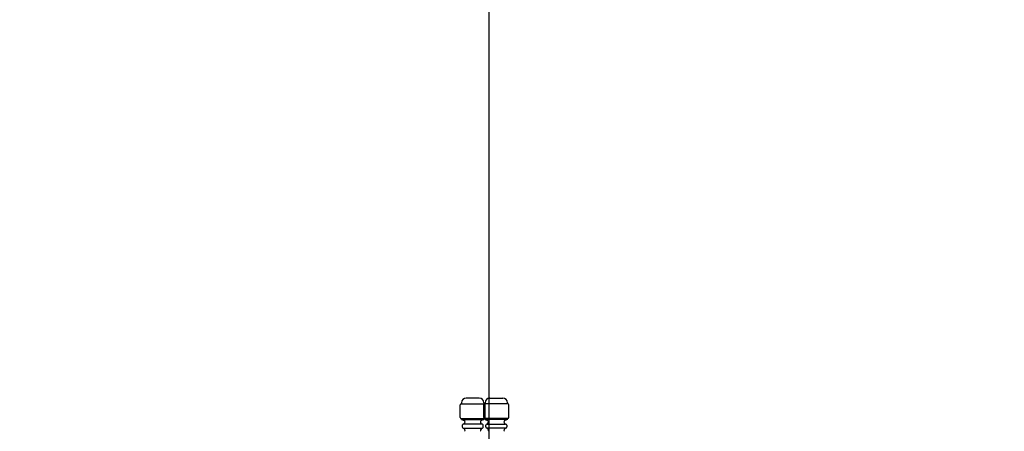
# Model space of a CAD drawing. Units: inches. Extents: x 2278 to 7495, y -71 to 1198.
# Tile 15 of 44: x 4938 to 5007, y 162 to 191. Entities that reach past the tile are written whole.
import ezdxf

# ---------------------------------------------------------------- set-up
doc = ezdxf.new("R2010")
doc.units = ezdxf.units.IN
doc.header["$MEASUREMENT"] = 0
doc.layers.add('A-ANNO-DIMS', color=2, linetype='Continuous', lineweight=18)
doc.layers.add('A-ELEV', color=7, linetype='Continuous', lineweight=25)
doc.styles.get("Standard").update_dxf_attribs({"font": 'arial.ttf'})
doc.dimstyles.get("Standard").update_dxf_attribs({"dimtxt": 6, "dimasz": 3, "dimexe": 0.18, "dimexo": 0.0625, "dimgap": 0.09, "dimtad": 0, "dimtih": 1, "dimtoh": 1, "dimdec": 0, "dimzin": 0, "dimdsep": 46, "dimlunit": 3, "dimtxsty": 'Standard', "dimblk": 'ARCHTICK', "dimcen": 0.09, "dimadec": 0, "dimazin": 0, "dimtfac": 1, "dimtdec": 0, "dimtofl": 0, "dimtmove": 0, "dimatfit": 3, "dimfxl": 1, "dimtolj": 1, "dimtzin": 0, "dimarcsym": 0})

# ---------------------------------------------------------------- blocks, each defined once
blk = doc.blocks.new('_ArchTick')
at = {"color": 0, "linetype": 'ByBlock', "const_width": 0.15}
blk.add_lwpolyline([(-0.5, -0.5), (0.5, 0.5)], dxfattribs=at)
blk = doc.blocks.new('*D123')
at = {"layer": 'A-ANNO-DIMS', "color": 0, "lineweight": -2, "transparency": 16777216}
for p, q in [((4736.95, 340.157), (4736.95, -23.427)), ((5145.676, -1.81), (5145.676, -23.427)), ((4736.95, -23.247), (4923.929, -23.247)), ((5145.676, -23.247), (4958.697, -23.247))]:
    blk.add_line(p, q, dxfattribs=at)
at = {"layer": 'Defpoints', "color": 0, "transparency": 16777216}
for p in [(4736.95, 340.219), (5145.676, -1.747), (5145.676, -23.247)]:
    blk.add_point(p, dxfattribs=at)
at = {"layer": 'A-ANNO-DIMS', "color": 0, "lineweight": -2, "transparency": 16777216, "xscale": 3, "yscale": 3, "zscale": 3, "rotation": 180}
blk.add_blockref('_ArchTick', (4736.95, -23.247), dxfattribs=at)
at = {"layer": 'A-ANNO-DIMS', "color": 0, "lineweight": -2, "transparency": 16777216, "xscale": 3, "yscale": 3, "zscale": 3}
blk.add_blockref('_ArchTick', (5145.676, -23.247), dxfattribs=at)
at = {"layer": 'A-ANNO-DIMS', "color": 0, "transparency": 16777216, "insert": (4941.313, -23.247), "char_height": 6, "attachment_point": 5}
blk.add_mtext('\\A1;34\'-0 1/2"', dxfattribs=at)
blk = doc.blocks.new('*D128')
at = {"layer": 'A-ANNO-DIMS', "color": 0, "lineweight": -2, "transparency": 16777216}
for p, q in [((4909.676, 99.315), (4909.676, 361.899)), ((4909.676, 361.719), (4932.111, 361.719)), ((4970.676, 361.719), (4948.241, 361.719)), ((4970.676, 60.779), (4970.676, 361.899))]:
    blk.add_line(p, q, dxfattribs=at)
at = {"layer": 'Defpoints', "color": 0, "transparency": 16777216}
for p in [(4970.676, 361.719), (4909.676, 99.253), (4970.676, 60.717)]:
    blk.add_point(p, dxfattribs=at)
at = {"layer": 'A-ANNO-DIMS', "color": 0, "lineweight": -2, "transparency": 16777216, "xscale": 3, "yscale": 3, "zscale": 3, "rotation": 180}
blk.add_blockref('_ArchTick', (4909.676, 361.719), dxfattribs=at)
at = {"layer": 'A-ANNO-DIMS', "color": 0, "lineweight": -2, "transparency": 16777216, "xscale": 3, "yscale": 3, "zscale": 3}
blk.add_blockref('_ArchTick', (4970.676, 361.719), dxfattribs=at)
at = {"layer": 'A-ANNO-DIMS', "color": 0, "transparency": 16777216, "insert": (4940.176, 361.719), "char_height": 6, "attachment_point": 5}
blk.add_mtext('\\A1;5\'-1"', dxfattribs=at)
blk = doc.blocks.new('*D129')
at = {"layer": 'A-ANNO-DIMS', "color": 0, "lineweight": -2, "transparency": 16777216}
for p, q in [((4970.676, 60.779), (4970.676, 361.899)), ((4970.676, 361.719), (4978.373, 361.719)), ((5016.176, 361.719), (5008.479, 361.719)), ((5016.176, 99.315), (5016.176, 361.899))]:
    blk.add_line(p, q, dxfattribs=at)
at = {"layer": 'Defpoints', "color": 0, "transparency": 16777216}
for p in [(5016.176, 361.719), (5016.176, 99.253), (4970.676, 60.717)]:
    blk.add_point(p, dxfattribs=at)
at = {"layer": 'A-ANNO-DIMS', "color": 0, "lineweight": -2, "transparency": 16777216, "xscale": 3, "yscale": 3, "zscale": 3, "rotation": 180}
blk.add_blockref('_ArchTick', (4970.676, 361.719), dxfattribs=at)
at = {"layer": 'A-ANNO-DIMS', "color": 0, "lineweight": -2, "transparency": 16777216, "xscale": 3, "yscale": 3, "zscale": 3}
blk.add_blockref('_ArchTick', (5016.176, 361.719), dxfattribs=at)
at = {"layer": 'A-ANNO-DIMS', "color": 0, "transparency": 16777216, "insert": (4993.426, 361.719), "char_height": 6, "attachment_point": 5}
blk.add_mtext('\\A1;3\'-9 1/2"', dxfattribs=at)

msp = doc.modelspace()

# ---------------------------------------------------------------- linework, layer by layer
at = {"layer": 'A-ELEV'}
for p, q in [((4970.676, 160.253), (4970.676, 244.253)), ((4969.988, 164.449), (4969.066, 164.449)), ((4970.724, 164.449), (4971.646, 164.449)), ((4968.641, 163.092), (4968.641, 163.965)), ((4968.722, 164.046), (4970.332, 164.046)), ((4968.737, 164.122), (4968.737, 164.046)), ((4970.298, 163.092), (4970.298, 163.965)), ((4970.318, 164.122), (4970.318, 164.046)), ((4971.989, 164.046), (4970.38, 164.046)), ((4970.394, 164.122), (4970.394, 164.046)), ((4970.414, 163.092), (4970.414, 163.965)), ((4971.975, 164.122), (4971.975, 164.046)), ((4972.071, 163.092), (4972.071, 163.965)), ((4968.722, 163.01), (4970.332, 163.01)), ((4968.737, 162.934), (4968.737, 163.01)), ((4968.737, 162.934), (4968.962, 162.837)), ((4968.737, 162.934), (4970.318, 162.934)), ((4970.318, 162.934), (4970.093, 162.837)), ((4970.318, 162.934), (4970.318, 163.01)), ((4971.989, 163.01), (4970.38, 163.01)), ((4970.394, 162.934), (4970.394, 163.01)), ((4970.394, 162.934), (4970.619, 162.837)), ((4971.975, 162.934), (4970.394, 162.934)), ((4971.975, 162.934), (4971.75, 162.837)), ((4971.975, 162.934), (4971.975, 163.01)), ((4968.876, 162.615), (4968.962, 162.711)), ((4968.876, 162.334), (4968.962, 162.238)), ((4970.179, 162.615), (4970.093, 162.711)), ((4970.179, 162.334), (4970.093, 162.238)), ((4970.451, 162.416), (4970.451, 162.533)), ((4970.533, 162.615), (4970.619, 162.711)), ((4970.533, 162.615), (4971.836, 162.615)), ((4970.533, 162.334), (4970.619, 162.238)), ((4971.836, 162.334), (4970.533, 162.334)), ((4971.836, 162.615), (4971.75, 162.711)), ((4971.836, 162.334), (4971.75, 162.238)), ((4971.918, 162.533), (4971.918, 162.416))]:
    msp.add_line(p, q, dxfattribs=at)
msp.add_lwpolyline([(4970.179, 162.615), (4968.876, 162.615, 0.414214), (4968.794, 162.533), (4968.794, 162.416, 0.414214), (4968.876, 162.334), (4970.179, 162.334, 0.414214), (4970.261, 162.416), (4970.261, 162.533, 0.414214)], format="xyb", close=True, dxfattribs=at)
for centre, radius, start, end in [((4969.089, 164.097), 0.352, 93.62058, 175.89193), ((4969.966, 164.097), 0.352, 4.10807, 86.37942), ((4970.746, 164.097), 0.352, 93.62058, 175.89193), ((4971.623, 164.097), 0.352, 4.10807, 86.37942), ((4968.722, 163.965), 0.0815, 90, 180), ((4970.38, 163.965), 0.0815, 90, 180), ((4970.332, 163.965), 0.0815, 0, 90), ((4971.989, 163.965), 0.0815, 0, 90), ((4968.722, 163.092), 0.0815, 180, 270), ((4968.91, 162.774), 0.0815, 309.328, 50.672), ((4970.145, 162.774), 0.0815, 129.328, 230.672), ((4970.38, 163.092), 0.0815, 180, 270), ((4970.332, 163.092), 0.0815, 270, 0), ((4970.567, 162.774), 0.0815, 309.328, 50.672), ((4971.802, 162.774), 0.0815, 129.328, 230.672), ((4971.989, 163.092), 0.0815, 270, 0), ((4968.91, 162.175), 0.0815, 309.328, 50.672), ((4970.145, 162.175), 0.0815, 129.328, 230.672), ((4970.533, 162.533), 0.0815, 90, 180), ((4970.533, 162.416), 0.0815, 180, 270), ((4970.567, 162.175), 0.0815, 309.328, 50.672), ((4971.802, 162.175), 0.0815, 129.328, 230.672), ((4971.836, 162.533), 0.0815, 0, 90), ((4971.836, 162.416), 0.0815, 270, 360)]:
    msp.add_arc(centre, radius, start, end, dxfattribs=at)

# ---------------------------------------------------------------- dimensions: what is measured, and where the dimension line sits
at = {"layer": 'A-ANNO-DIMS'}
for base, p1, p2, picture, middle in [((5016.176, 361.719), (4970.676, 60.717), (5016.176, 99.253), '*D129', (4993.426, 361.719)), ((4970.676, 361.719), (4909.676, 99.253), (4970.676, 60.717), '*D128', (4940.176, 361.719)), ((5145.676, -23.247), (4736.95, 340.219), (5145.676, -1.747), '*D123', (4941.313, -23.247))]:
    dim = msp.add_linear_dim(base=base, p1=p1, p2=p2, dimstyle='Standard', override={"dimdec": 1, "dimlfac": 1, "dimrnd": 0, "dimzin": 1, "dimdsep": 46, "dimlunit": 4, "dimfrac": 2}, dxfattribs=at)
    dim.commit()
    dim.dimension.update_dxf_attribs({"geometry": picture, "text_midpoint": middle})

doc.saveas('drawing.dxf')
